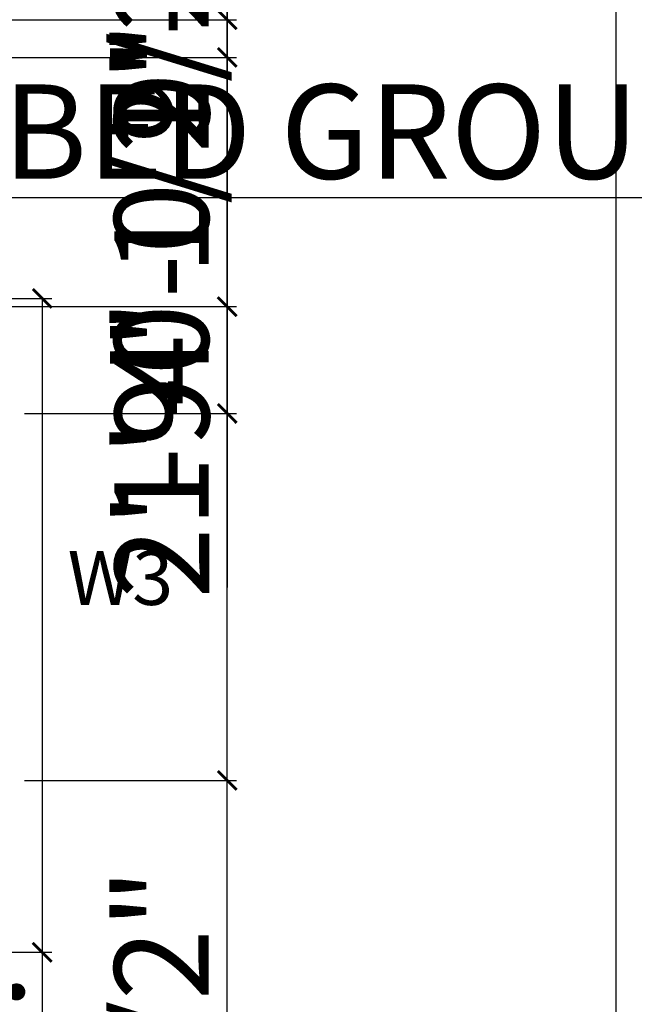
# Model space of a CAD drawing. Units: inches. Extents: x 1763 to 2368, y 1500 to 2097.
# Tile 22 of 24: x 2189 to 2271, y 1856 to 1986. Entities that reach past the tile are written whole.
import ezdxf

# ---------------------------------------------------------------- set-up
doc = ezdxf.new("R2010")
doc.units = ezdxf.units.IN
doc.layers.add('A-ANNO-DIMS', color=2, linetype='Continuous', lineweight=18)
doc.layers.add('A-ANNO-TEXT', color=7, linetype='Continuous', lineweight=18)
doc.styles.get("Standard").update_dxf_attribs({"font": 'arial.ttf'})
doc.dimstyles.new('ISO-25', dxfattribs={"dimtxt": 12.5, "dimasz": 2.5, "dimexe": 1.25, "dimexo": 0.625, "dimtad": 1, "dimdec": 0, "dimlunit": 4, "dimtxsty": 'Standard', "dimblk": 'ARCHTICK', "dimcen": 2.5, "dimclrd": 3, "dimclrt": 4, "dimadec": 0, "dimazin": 0, "dimtfac": 1, "dimtdec": 0, "dimtmove": 0, "dimatfit": 3, "dimfxl": 1, "dimarcsym": 0})

# ---------------------------------------------------------------- blocks, each defined once
blk = doc.blocks.new('_ArchTick')
at = {"color": 0, "linetype": 'ByBlock', "const_width": 0.15}
blk.add_lwpolyline([(-0.5, -0.5), (0.5, 0.5)], dxfattribs=at)
blk = doc.blocks.new('*D22')
at = {"layer": 'A-ANNO-DIMS', "color": 0, "lineweight": -2, "transparency": 16777216}
for p, q in [((2189.72, 2043.27), (2269.32, 2043.27)), ((2268.07, 2043.27), (2268.07, 1563.27)), ((2189.72, 1563.27), (2269.32, 1563.27))]:
    blk.add_line(p, q, dxfattribs=at)
at = {"layer": 'Defpoints', "color": 0, "transparency": 16777216}
for p in [(2189.09, 2043.27), (2189.09, 1563.27), (2268.07, 1563.27)]:
    blk.add_point(p, dxfattribs=at)
at = {"layer": 'A-ANNO-DIMS', "color": 0, "lineweight": -2, "transparency": 16777216, "xscale": 2.5, "yscale": 2.5, "zscale": 2.5}
for p, rotation in [((2268.07, 2043.27), 90), ((2268.07, 1563.27), 270)]:
    blk.add_blockref('_ArchTick', p, dxfattribs=dict(at, rotation=rotation))
at = {"layer": 'A-ANNO-DIMS', "color": 0, "transparency": 16777216, "insert": (2261.06, 1803.27), "char_height": 12.5, "attachment_point": 5, "rotation": 90}
blk.add_mtext("40'", dxfattribs=at)
blk = doc.blocks.new('*D23')
at = {"layer": 'A-ANNO-DIMS', "color": 0, "lineweight": -2, "transparency": 16777216}
for p, q in [((2089.48, 1949.98), (2089.48, 1963.99)), ((2178.7, 1949.98), (2178.7, 1963.99))]:
    blk.add_line(p, q, dxfattribs=at)
at = {"layer": 'A-ANNO-DIMS', "color": 3, "lineweight": -2, "transparency": 16777216}
for p, q in [((2089.48, 1962.74), (2178.7, 1962.74)), ((2178.7, 1962.74), (2367.73, 1962.74))]:
    blk.add_line(p, q, dxfattribs=at)
at = {"layer": 'Defpoints', "color": 0, "transparency": 16777216}
for p in [(2178.7, 1962.74), (2089.48, 1949.35), (2178.7, 1949.35)]:
    blk.add_point(p, dxfattribs=at)
at = {"layer": 'A-ANNO-DIMS', "color": 3, "lineweight": -2, "transparency": 16777216, "xscale": 2.5, "yscale": 2.5, "zscale": 2.5, "rotation": 180}
blk.add_blockref('_ArchTick', (2089.48, 1962.74), dxfattribs=at)
at = {"layer": 'A-ANNO-DIMS', "color": 3, "lineweight": -2, "transparency": 16777216, "xscale": 2.5, "yscale": 2.5, "zscale": 2.5}
blk.add_blockref('_ArchTick', (2178.7, 1962.74), dxfattribs=at)
at = {"layer": 'A-ANNO-DIMS', "color": 4, "transparency": 16777216, "insert": (2274.46, 1969.83), "char_height": 12.5, "attachment_point": 5}
blk.add_mtext('BED GROUP 7\'-5" TYP.', dxfattribs=at)
blk = doc.blocks.new('*D24')
at = {"layer": 'A-ANNO-DIMS', "color": 0, "lineweight": -2, "transparency": 16777216}
for p, q in [((2179.32, 1949.35), (2193.33, 1949.35)), ((2179.32, 1862.76), (2193.33, 1862.76))]:
    blk.add_line(p, q, dxfattribs=at)
at = {"layer": 'A-ANNO-DIMS', "color": 3, "lineweight": -2, "transparency": 16777216}
for p, q in [((2192.08, 1949.35), (2192.08, 1862.76)), ((2192.08, 1862.76), (2192.08, 1753.79))]:
    blk.add_line(p, q, dxfattribs=at)
at = {"layer": 'Defpoints', "color": 0, "transparency": 16777216}
for p in [(2178.7, 1949.35), (2178.7, 1862.76), (2192.08, 1862.76)]:
    blk.add_point(p, dxfattribs=at)
at = {"layer": 'A-ANNO-DIMS', "color": 3, "lineweight": -2, "transparency": 16777216, "xscale": 2.5, "yscale": 2.5, "zscale": 2.5}
for p, rotation in [((2192.08, 1949.35), 90), ((2192.08, 1862.76), 270)]:
    blk.add_blockref('_ArchTick', p, dxfattribs=dict(at, rotation=rotation))
at = {"layer": 'A-ANNO-DIMS', "color": 4, "transparency": 16777216, "insert": (2184.99, 1807.02), "char_height": 12.5, "attachment_point": 5, "rotation": 90}
blk.add_mtext('7\'-2 1/2" TYP.', dxfattribs=at)
blk = doc.blocks.new('*D54')
at = {"layer": 'A-ANNO-DIMS', "color": 0, "lineweight": -2, "transparency": 16777216}
for p, q in [((2189.72, 1885.52), (2217.84, 1885.52)), ((2189.72, 1795.26), (2217.84, 1795.26))]:
    blk.add_line(p, q, dxfattribs=at)
at = {"layer": 'A-ANNO-DIMS', "color": 3, "lineweight": -2, "transparency": 16777216}
blk.add_line((2216.59, 1795.26), (2216.59, 1885.52), dxfattribs=at)
at = {"layer": 'Defpoints', "color": 0, "transparency": 16777216}
for p in [(2189.09, 1885.52), (2216.59, 1885.52), (2189.09, 1795.26)]:
    blk.add_point(p, dxfattribs=at)
at = {"layer": 'A-ANNO-DIMS', "color": 3, "lineweight": -2, "transparency": 16777216, "xscale": 2.5, "yscale": 2.5, "zscale": 2.5}
for p, rotation in [((2216.59, 1885.52), 90), ((2216.59, 1795.26), 270)]:
    blk.add_blockref('_ArchTick', p, dxfattribs=dict(at, rotation=rotation))
at = {"layer": 'A-ANNO-DIMS', "color": 4, "transparency": 16777216, "insert": (2209.5, 1840.39), "char_height": 12.5, "attachment_point": 5, "rotation": 90}
blk.add_mtext('7\'-6 1/2"', dxfattribs=at)
blk = doc.blocks.new('*D55')
at = {"layer": 'A-ANNO-DIMS', "color": 3, "lineweight": -2, "transparency": 16777216}
for p, q in [((2216.59, 1934.11), (2216.59, 2000.72)), ((2216.59, 1885.52), (2216.59, 1934.11))]:
    blk.add_line(p, q, dxfattribs=at)
at = {"layer": 'A-ANNO-DIMS', "color": 0, "lineweight": -2, "transparency": 16777216}
for p, q in [((2189.72, 1934.11), (2217.84, 1934.11)), ((2189.72, 1885.52), (2217.84, 1885.52))]:
    blk.add_line(p, q, dxfattribs=at)
at = {"layer": 'Defpoints', "color": 0, "transparency": 16777216}
for p in [(2189.09, 1934.11), (2216.59, 1934.11), (2189.09, 1885.52)]:
    blk.add_point(p, dxfattribs=at)
at = {"layer": 'A-ANNO-DIMS', "color": 3, "lineweight": -2, "transparency": 16777216, "xscale": 2.5, "yscale": 2.5, "zscale": 2.5}
for p, rotation in [((2216.59, 1934.11), 90), ((2216.59, 1885.52), 270)]:
    blk.add_blockref('_ArchTick', p, dxfattribs=dict(at, rotation=rotation))
at = {"layer": 'A-ANNO-DIMS', "color": 4, "transparency": 16777216, "insert": (2209.5, 1968.66), "char_height": 12.5, "attachment_point": 5, "rotation": 90}
blk.add_mtext('4\'-0 1/2"', dxfattribs=at)
blk = doc.blocks.new('*D56')
at = {"layer": 'A-ANNO-DIMS', "color": 0, "lineweight": -2, "transparency": 16777216}
for p, q in [((2189.72, 2043.27), (2217.84, 2043.27)), ((2189.72, 1934.11), (2217.84, 1934.11))]:
    blk.add_line(p, q, dxfattribs=at)
at = {"layer": 'A-ANNO-DIMS', "color": 3, "lineweight": -2, "transparency": 16777216}
blk.add_line((2216.59, 1934.11), (2216.59, 2043.27), dxfattribs=at)
at = {"layer": 'Defpoints', "color": 0, "transparency": 16777216}
for p in [(2189.09, 2043.27), (2216.59, 2043.27), (2189.09, 1934.11)]:
    blk.add_point(p, dxfattribs=at)
at = {"layer": 'A-ANNO-DIMS', "color": 3, "lineweight": -2, "transparency": 16777216, "xscale": 2.5, "yscale": 2.5, "zscale": 2.5}
for p, rotation in [((2216.59, 2043.27), 90), ((2216.59, 1934.11), 270)]:
    blk.add_blockref('_ArchTick', p, dxfattribs=dict(at, rotation=rotation))
at = {"layer": 'A-ANNO-DIMS', "color": 4, "transparency": 16777216, "insert": (2209.58, 1988.69), "char_height": 12.5, "attachment_point": 5, "rotation": 90}
blk.add_mtext('9\'-1"', dxfattribs=at)
blk = doc.blocks.new('*D63')
at = {"layer": 'A-ANNO-DIMS', "color": 0, "lineweight": -2, "transparency": 16777216}
for p, q in [((2120.61, 1981.9), (2120.61, 2072.02)), ((2166.28, 1981.9), (2166.28, 2072.02))]:
    blk.add_line(p, q, dxfattribs=at)
at = {"layer": 'A-ANNO-DIMS', "color": 3, "lineweight": -2, "transparency": 16777216}
for p, q in [((2120.61, 2070.77), (2166.28, 2070.77)), ((2166.28, 2070.77), (2232.38, 2070.77))]:
    blk.add_line(p, q, dxfattribs=at)
at = {"layer": 'Defpoints', "color": 0, "transparency": 16777216}
for p in [(2166.28, 2070.77), (2120.61, 1981.27), (2166.28, 1981.27)]:
    blk.add_point(p, dxfattribs=at)
at = {"layer": 'A-ANNO-DIMS', "color": 3, "lineweight": -2, "transparency": 16777216, "xscale": 2.5, "yscale": 2.5, "zscale": 2.5, "rotation": 180}
blk.add_blockref('_ArchTick', (2120.61, 2070.77), dxfattribs=at)
at = {"layer": 'A-ANNO-DIMS', "color": 3, "lineweight": -2, "transparency": 16777216, "xscale": 2.5, "yscale": 2.5, "zscale": 2.5}
blk.add_blockref('_ArchTick', (2166.28, 2070.77), dxfattribs=at)
at = {"layer": 'A-ANNO-DIMS', "color": 4, "transparency": 16777216, "insert": (2200.58, 2077.87), "char_height": 12.5, "attachment_point": 5}
blk.add_mtext('3\'-9 1/2"', dxfattribs=at)
blk = doc.blocks.new('*D78')
at = {"layer": 'A-ANNO-DIMS', "color": 0, "lineweight": -2, "transparency": 16777216}
for p, q in [((1996.72, 1981.27), (2217.84, 1981.27)), ((1986.22, 1948.27), (2217.84, 1948.27))]:
    blk.add_line(p, q, dxfattribs=at)
at = {"layer": 'A-ANNO-DIMS', "color": 3, "lineweight": -2, "transparency": 16777216}
for p, q in [((2216.59, 1981.27), (2216.59, 1948.27)), ((2216.59, 1948.27), (2216.59, 1911.08))]:
    blk.add_line(p, q, dxfattribs=at)
at = {"layer": 'Defpoints', "color": 0, "transparency": 16777216}
for p in [(1996.09, 1981.27), (1985.59, 1948.27), (2216.59, 1948.27)]:
    blk.add_point(p, dxfattribs=at)
at = {"layer": 'A-ANNO-DIMS', "color": 3, "lineweight": -2, "transparency": 16777216, "xscale": 2.5, "yscale": 2.5, "zscale": 2.5}
for p, rotation in [((2216.59, 1981.27), 90), ((2216.59, 1948.27), 270)]:
    blk.add_blockref('_ArchTick', p, dxfattribs=dict(at, rotation=rotation))
at = {"layer": 'A-ANNO-DIMS', "color": 4, "transparency": 16777216, "insert": (2209.58, 1928.43), "char_height": 12.5, "attachment_point": 5, "rotation": 90}
blk.add_mtext('2\'-9"', dxfattribs=at)
blk = doc.blocks.new('*D95')
at = {"layer": 'A-ANNO-DIMS', "color": 0, "lineweight": -2, "transparency": 16777216}
for p, q in [((2125.16, 1998.77), (2217.84, 1998.77)), ((2121.24, 1986.27), (2217.84, 1986.27))]:
    blk.add_line(p, q, dxfattribs=at)
at = {"layer": 'A-ANNO-DIMS', "color": 3, "lineweight": -2, "transparency": 16777216}
for p, q in [((2216.59, 1998.77), (2216.59, 1986.27)), ((2216.59, 1986.27), (2216.59, 1921.34))]:
    blk.add_line(p, q, dxfattribs=at)
at = {"layer": 'Defpoints', "color": 0, "transparency": 16777216}
for p in [(2124.53, 1998.77), (2120.61, 1986.27), (2216.59, 1986.27)]:
    blk.add_point(p, dxfattribs=at)
at = {"layer": 'A-ANNO-DIMS', "color": 3, "lineweight": -2, "transparency": 16777216, "xscale": 2.5, "yscale": 2.5, "zscale": 2.5}
for p, rotation in [((2216.59, 1998.77), 90), ((2216.59, 1986.27), 270)]:
    blk.add_blockref('_ArchTick', p, dxfattribs=dict(at, rotation=rotation))
at = {"layer": 'A-ANNO-DIMS', "color": 4, "transparency": 16777216, "insert": (2209.5, 1952.56), "char_height": 12.5, "attachment_point": 5, "rotation": 90}
blk.add_mtext('1\'-0 1/2"', dxfattribs=at)

msp = doc.modelspace()

# ---------------------------------------------------------------- texts
at = {"layer": 'A-ANNO-TEXT'}
msp.add_text('W3', height=7.155, dxfattribs=at).set_placement((2195.44, 1908.76))

# ---------------------------------------------------------------- dimensions: what is measured, and where the dimension line sits
at = {"layer": 'A-ANNO-DIMS'}
dim = msp.add_linear_dim(base=(2166.28, 2070.77), p1=(2120.61, 1981.27), p2=(2166.28, 1981.27), dimstyle='ISO-25', override={"dimdec": 1, "dimlfac": 1, "dimrnd": 0, "dimzin": 1, "dimdsep": 46, "dimlunit": 4, "dimfrac": 2}, dxfattribs=at)
dim.commit()
dim.dimension.update_dxf_attribs({"geometry": '*D63', "text_midpoint": (2200.58, 2077.87)})
for base, p1, p2, override, picture, middle in [((2268.07, 1563.27), (2189.09, 2043.27), (2189.09, 1563.27), {"dimclrd": 0, "dimclre": 0, "dimclrt": 0}, '*D22', (2261.06, 1803.27)), ((2216.59, 2043.27), (2189.09, 1934.11), (2189.09, 2043.27), {"dimdec": 1, "dimlfac": 1, "dimrnd": 0, "dimzin": 1, "dimdsep": 46, "dimlunit": 4, "dimfrac": 2}, '*D56', (2209.58, 1988.69)), ((2216.59, 1934.11), (2189.09, 1885.52), (2189.09, 1934.11), {"dimdec": 1, "dimlfac": 1, "dimrnd": 0, "dimzin": 1, "dimdsep": 46, "dimlunit": 4, "dimfrac": 2}, '*D55', (2209.5, 1968.66)), ((2216.59, 1986.27), (2124.53, 1998.77), (2120.61, 1986.27), {"dimdec": 1, "dimlfac": 1, "dimrnd": 0, "dimzin": 1, "dimdsep": 46, "dimlunit": 4, "dimfrac": 2}, '*D95', (2209.5, 1952.56)), ((2216.59, 1948.27), (1996.09, 1981.27), (1985.59, 1948.27), {"dimdec": 1, "dimlfac": 1, "dimrnd": 0, "dimzin": 1, "dimdsep": 46, "dimlunit": 4, "dimfrac": 2}, '*D78', (2209.58, 1928.43)), ((2216.59, 1885.52), (2189.09, 1795.26), (2189.09, 1885.52), {"dimdec": 1, "dimlfac": 1, "dimrnd": 0, "dimzin": 1, "dimdsep": 46, "dimlunit": 4, "dimfrac": 2}, '*D54', (2209.5, 1840.39))]:
    dim = msp.add_linear_dim(base=base, p1=p1, p2=p2, angle=90, dimstyle='ISO-25', override=override, dxfattribs=at)
    dim.commit()
    dim.dimension.update_dxf_attribs({"geometry": picture, "text_midpoint": middle})
dim = msp.add_linear_dim(base=(2178.7, 1962.74), p1=(2089.48, 1949.35), p2=(2178.7, 1949.35), text='BED GROUP <> TYP.', dimstyle='ISO-25', override={"dimdec": 1, "dimlfac": 1, "dimrnd": 0, "dimzin": 1, "dimdsep": 46, "dimlunit": 4, "dimfrac": 2}, dxfattribs=at)
dim.commit()
dim.dimension.update_dxf_attribs({"geometry": '*D23', "text_midpoint": (2274.46, 1969.83)})
dim = msp.add_linear_dim(base=(2192.08, 1862.76), p1=(2178.7, 1949.35), p2=(2178.7, 1862.76), angle=270, text='<> TYP.', dimstyle='ISO-25', override={"dimdec": 1, "dimlfac": 1, "dimrnd": 0, "dimzin": 1, "dimdsep": 46, "dimlunit": 4, "dimfrac": 2}, dxfattribs=at)
dim.commit()
dim.dimension.update_dxf_attribs({"geometry": '*D24', "text_midpoint": (2184.99, 1807.02)})

doc.saveas('drawing.dxf')
